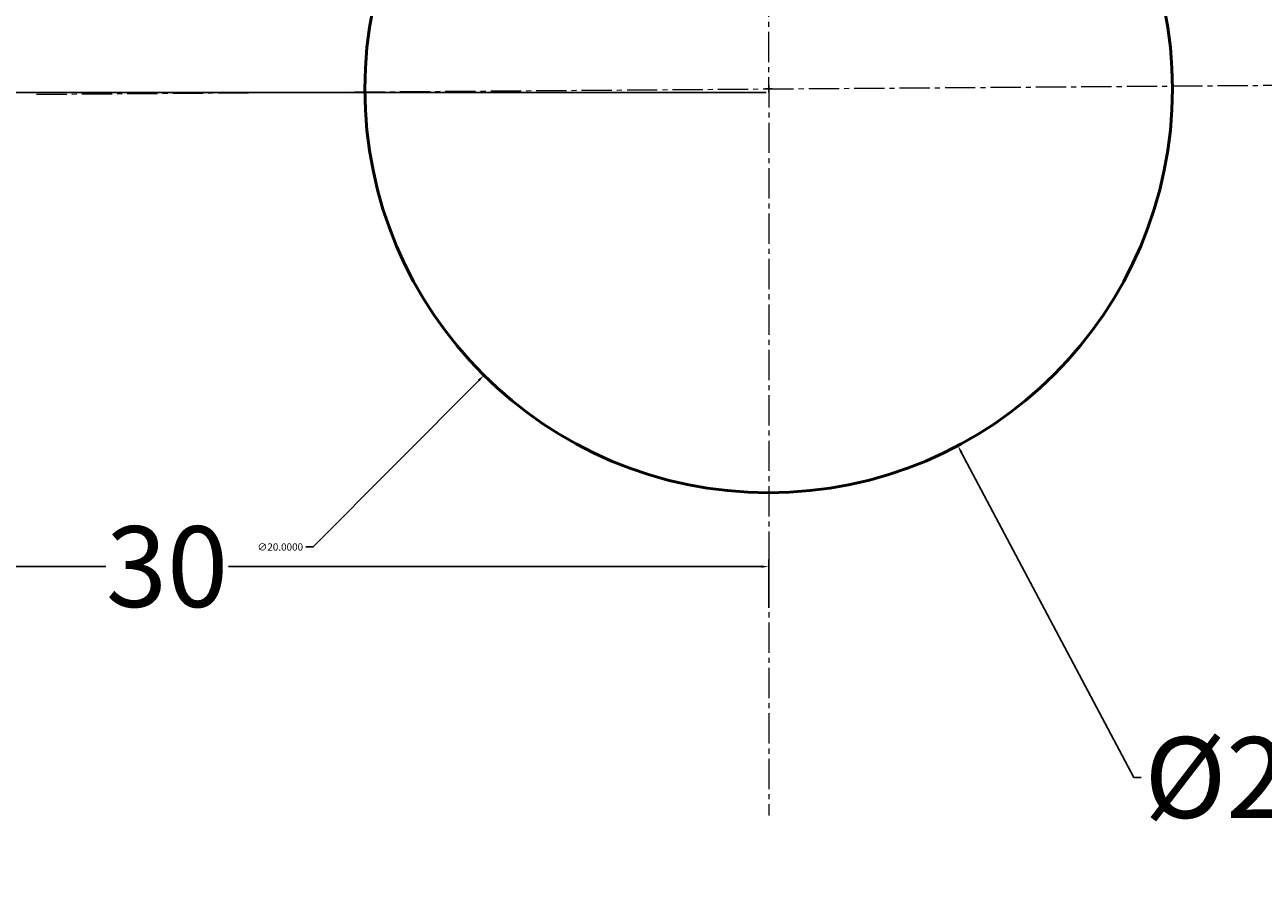
# Model space of a CAD drawing. Units: millimetres. Extents: x -60 to 113, y -37 to 126.
# Tile 10 of 17: x 19 to 49, y 27 to 48. Entities that reach past the tile are written whole.
import ezdxf

# ---------------------------------------------------------------- set-up
doc = ezdxf.new("R2010")
doc.units = ezdxf.units.MM
doc.header["$MEASUREMENT"] = 0
doc.linetypes.add('CENTER2', pattern=[1.125, 0.75, -0.125, 0.125, -0.125])
for name, color, linetype, lineweight in [('M-CNTR', 4, 'CENTER2', 18), ('M-DIMS', 2, 'Continuous', 25), ('M-OUTL', 7, 'Continuous', 50)]:
    doc.layers.add(name, color=color, linetype=linetype, lineweight=lineweight)
doc.styles.get("Standard").update_dxf_attribs({"font": 'arial.ttf'})
doc.dimstyles.get("Standard").update_dxf_attribs({"dimtxt": 0.18, "dimasz": 0.18, "dimexe": 0.18, "dimexo": 0.0625, "dimgap": 0.09, "dimtad": 0, "dimtih": 1, "dimtoh": 1, "dimdec": 4, "dimzin": 0, "dimdsep": 46, "dimtxsty": 'Standard', "dimcen": 0.09, "dimadec": 0, "dimazin": 0, "dimtfac": 1, "dimtdec": 4, "dimtofl": 0, "dimtmove": 0, "dimatfit": 3, "dimfxl": 1, "dimtolj": 1, "dimtzin": 0, "dimarcsym": 0})

# ---------------------------------------------------------------- blocks, each defined once
blk = doc.blocks.new('*D11')
at = {"layer": 'Defpoints', "color": 0, "transparency": 16777216}
for p in [(32.38, 55.737), (41.75, 38.068)]:
    blk.add_point(p, dxfattribs=at)
at = {"layer": 'M-DIMS', "color": 0, "lineweight": -2, "transparency": 16777216}
for p, q in [((37.065, 46.813), (37.065, 46.993)), ((36.975, 46.903), (37.155, 46.903)), ((46.107, 29.851), (41.834, 37.909)), ((46.287, 29.851), (46.107, 29.851))]:
    blk.add_line(p, q, dxfattribs=at)
at = {"layer": 'M-DIMS', "color": 0, "transparency": 16777216}
blk.add_solid([(41.861, 37.923), (41.808, 37.895), (41.75, 38.068)], dxfattribs=at)
at = {"layer": 'M-DIMS', "color": 0, "transparency": 16777216, "insert": (48.894, 29.851), "char_height": 0.18, "attachment_point": 5}
blk.add_mtext('\\A1;{\\H11.11111x;%%C20}', dxfattribs=at)
blk = doc.blocks.new('*D13')
at = {"layer": 'Defpoints', "color": 0, "transparency": 16777216}
for p in [(37.065, 46.813), (-39.303, 6.903), (7.267, 6.903)]:
    blk.add_point(p, dxfattribs=at)
at = {"layer": 'M-DIMS', "color": 0, "lineweight": -2, "transparency": 16777216}
for p, q in [((37.002, 46.813), (-39.483, 46.813)), ((-39.303, 46.633), (-39.303, 27.969)), ((-39.303, 7.083), (-39.303, 25.747)), ((7.204, 6.903), (-39.483, 6.903))]:
    blk.add_line(p, q, dxfattribs=at)
at = {"layer": 'M-DIMS', "color": 0, "transparency": 16777216}
for points in [[(-39.333, 46.633), (-39.273, 46.633), (-39.303, 46.813)], [(-39.333, 7.083), (-39.273, 7.083), (-39.303, 6.903)]]:
    blk.add_solid(points, dxfattribs=at)
at = {"layer": 'M-DIMS', "color": 0, "transparency": 16777216, "insert": (-39.303, 26.858), "char_height": 0.18, "attachment_point": 5}
blk.add_mtext('\\A1;{\\H11.11111x;40}', dxfattribs=at)
blk = doc.blocks.new('*D17')
at = {"layer": 'Defpoints', "color": 0, "transparency": 16777216}
for p in [(67.355, 124.823), (10.532, 88.533), (67.355, 6.442)]:
    blk.add_point(p, dxfattribs=at)
at = {"layer": 'M-DIMS', "color": 0, "lineweight": -2, "transparency": 16777216}
for p, q in [((10.532, 88.595), (10.532, 125.003)), ((10.712, 124.823), (37.422, 124.823)), ((67.175, 124.823), (40.465, 124.823)), ((67.355, 6.504), (67.355, 125.003))]:
    blk.add_line(p, q, dxfattribs=at)
at = {"layer": 'M-DIMS', "color": 0, "transparency": 16777216}
for points in [[(10.712, 124.853), (10.712, 124.793), (10.532, 124.823)], [(67.175, 124.853), (67.175, 124.793), (67.355, 124.823)]]:
    blk.add_solid(points, dxfattribs=at)
at = {"layer": 'M-DIMS', "color": 0, "transparency": 16777216, "insert": (38.944, 124.823), "char_height": 0.18, "attachment_point": 5}
blk.add_mtext('\\A1;{\\H11.11111x;56}', dxfattribs=at)
blk = doc.blocks.new('*D18')
at = {"layer": 'Defpoints', "color": 0, "transparency": 16777216}
for p in [(37.067, 35.073), (7.267, 34.023), (37.067, 33.992)]:
    blk.add_point(p, dxfattribs=at)
at = {"layer": 'M-DIMS', "color": 0, "lineweight": -2, "transparency": 16777216}
for p, q in [((7.267, 34.085), (7.267, 35.253)), ((7.447, 35.073), (20.648, 35.073)), ((36.887, 35.073), (23.685, 35.073)), ((37.067, 34.055), (37.067, 35.253))]:
    blk.add_line(p, q, dxfattribs=at)
at = {"layer": 'M-DIMS', "color": 0, "transparency": 16777216}
for points in [[(7.447, 35.103), (7.447, 35.043), (7.267, 35.073)], [(36.887, 35.103), (36.887, 35.043), (37.067, 35.073)]]:
    blk.add_solid(points, dxfattribs=at)
at = {"layer": 'M-DIMS', "color": 0, "transparency": 16777216, "insert": (22.167, 35.073), "char_height": 0.18, "attachment_point": 5}
blk.add_mtext('\\A1;{\\H11.11111x;30}', dxfattribs=at)
blk = doc.blocks.new('*D23')
at = {"layer": 'Defpoints', "color": 0, "transparency": 16777216}
for p in [(44.117, 53.993), (30.013, 39.813)]:
    blk.add_point(p, dxfattribs=at)
at = {"layer": 'M-DIMS', "color": 0, "lineweight": -2, "transparency": 16777216}
for p, q in [((37.065, 46.813), (37.065, 46.993)), ((36.975, 46.903), (37.155, 46.903)), ((25.781, 35.559), (29.886, 39.685)), ((25.601, 35.559), (25.781, 35.559))]:
    blk.add_line(p, q, dxfattribs=at)
at = {"layer": 'M-DIMS', "color": 0, "transparency": 16777216}
blk.add_solid([(29.864, 39.706), (29.907, 39.664), (30.013, 39.813)], dxfattribs=at)
at = {"layer": 'M-DIMS', "color": 0, "transparency": 16777216, "insert": (24.97, 35.559), "char_height": 0.18, "attachment_point": 5}
blk.add_mtext('\\A1;∅20.0000', dxfattribs=at)

msp = doc.modelspace()

# ---------------------------------------------------------------- linework, layer by layer
at = {"layer": 'M-CNTR'}
for p, q in [((37.06129, 67.44095), (37.06756, 28.90573)), ((18.93276, 46.7704), (53.1925, 47.02024))]:
    msp.add_line(p, q, dxfattribs=at)
at = {"layer": 'M-OUTL'}
msp.add_circle((37.06463, 46.90263), 10, dxfattribs=at)
for centre, radius, start, end in [((-30.77517, 49.3506), 84, 356.2470441, 43.4253235), ((67.26481, 6.44179), 27, 215.384639, 96.582684)]:
    msp.add_arc(centre, radius, start, end, dxfattribs=at)

# ---------------------------------------------------------------- dimensions: what is measured, and where the dimension line sits
at = {"layer": 'M-DIMS'}
for base, p1, p2, text, picture, middle in [((67.35481, 124.82251), (10.53227, 88.53289), (67.35481, 6.44179), '{\\H11.11111x;56}', '*D17', (38.94354, 124.82251)), ((37.06673, 35.07294), (7.26659, 34.0227), (37.06673, 33.99249), '{\\H11.11111x;30}', '*D18', (22.16666, 35.07294))]:
    dim = msp.add_linear_dim(base=base, p1=p1, p2=p2, text=text, dimstyle='Standard', override={"dimclrd": 0, "dimclre": 0, "dimclrt": 0}, dxfattribs=at)
    dim.commit()
    dim.dimension.update_dxf_attribs({"geometry": picture, "text_midpoint": middle})
dim = msp.add_diameter_dim_2p(p1=(32.37959, 55.73724), p2=(41.74967, 38.06802), text='{\\H11.11111x;%%C20}', dimstyle='Standard', override={"dimclrd": 0, "dimclre": 0, "dimclrt": 0}, dxfattribs=at)
dim.commit()
dim.dimension.update_dxf_attribs({"geometry": '*D11', "text_midpoint": (48.8944, 29.85072), "dimtype": 163})
dim = msp.add_diameter_dim_2p(p1=(44.11671, 53.99263), p2=(30.01255, 39.81262), dimstyle='Standard', override={"dimdec": 4, "dimlfac": 1, "dimrnd": 0, "dimzin": 0, "dimdsep": 46, "dimlunit": 2}, dxfattribs=at)
dim.commit()
dim.dimension.update_dxf_attribs({"geometry": '*D23', "text_midpoint": (24.97014, 35.55862), "dimtype": 163})
dim = msp.add_linear_dim(base=(-39.30316, 6.9027), p1=(37.06463, 46.81263), p2=(7.26659, 6.9027), angle=90, text='{\\H11.11111x;40}', dimstyle='Standard', override={"dimclrd": 0, "dimclre": 0, "dimclrt": 0}, dxfattribs=at)
dim.commit()
dim.dimension.update_dxf_attribs({"geometry": '*D13', "text_midpoint": (-39.30316, 26.85766)})

doc.saveas('drawing.dxf')
